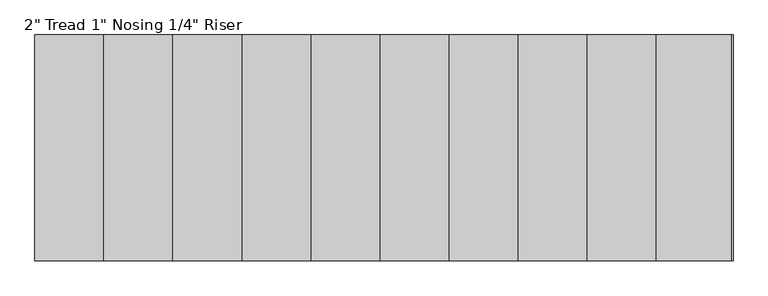
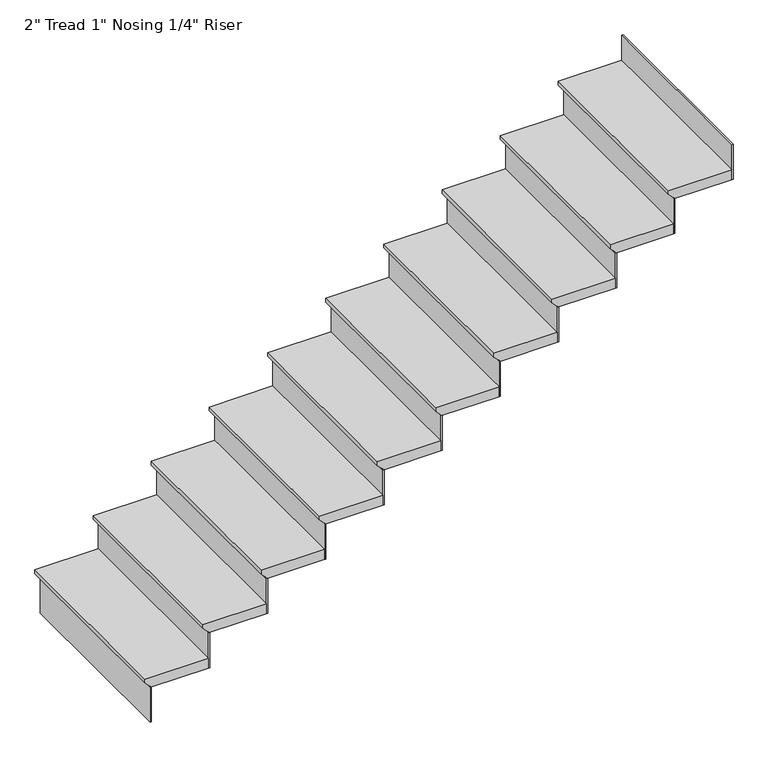
"""IFC4 building model written with IfcOpenShell, lengths in millimetres: stair flight geometry."""

from ifc_helpers import new_model, si_unit, frame, origin, place, context, project, spatial, polyline, outline, extrude, source, transform, mapped, element, save


def stair_flight_d3d59df2(model_context):
    return source(origin(), model_context, "Body", "SweptSolid", [
        extrude(outline(polyline([(1422.4, -12143.9167709), (1422.4, -12448.7167709), (1403.35, -12448.7167709), (1377.95, -12423.3167709), (1371.6, -12423.3167709), (1371.6, -12143.9167709), (1422.4, -12143.9167709)])), frame((0.0, 2766.6362133, 0.0), z_axis=(0.0, 1.0, 0.0), x_axis=(0.0, 0.0, 1.0)), (0.0, 0.0, 1.0), 914.4),
        extrude(outline(polyline([(-12416.9667709, 2766.6362133), (-12423.3167709, 2766.6362133), (-12423.3167709, 3681.0362133), (-12416.9667709, 3681.0362133), (-12416.9667709, 2766.6362133)])), frame((0.0, 0.0, 1193.8), z_axis=(0.0, 0.0, 1.0), x_axis=(1.0, 0.0, 0.0)), (0.0, 0.0, 1.0), 177.8),
        extrude(outline(polyline([(-12137.5667709, 2766.6362133), (-12143.9167709, 2766.6362133), (-12143.9167709, 3681.0362133), (-12137.5667709, 3681.0362133), (-12137.5667709, 2766.6362133)])), frame((0.0, 0.0, 1371.6), z_axis=(0.0, 0.0, 1.0), x_axis=(1.0, 0.0, 0.0)), (0.0, 0.0, 1.0), 177.8),
        extrude(outline(polyline([(1600.2, -11864.5167709), (1600.2, -12169.3167709), (1581.15, -12169.3167709), (1555.75, -12143.9167709), (1549.4, -12143.9167709), (1549.4, -11864.5167709), (1600.2, -11864.5167709)])), frame((0.0, 2766.6362133, 0.0), z_axis=(0.0, 1.0, 0.0), x_axis=(0.0, 0.0, 1.0)), (0.0, 0.0, 1.0), 914.4),
        extrude(outline(polyline([(-11858.1667709, 2766.6362133), (-11864.5167709, 2766.6362133), (-11864.5167709, 3681.0362133), (-11858.1667709, 3681.0362133), (-11858.1667709, 2766.6362133)])), frame((0.0, 0.0, 1549.4), z_axis=(0.0, 0.0, 1.0), x_axis=(1.0, 0.0, 0.0)), (0.0, 0.0, 1.0), 177.8),
        extrude(outline(polyline([(1778.0, -11585.1167709), (1778.0, -11889.9167709), (1758.95, -11889.9167709), (1733.55, -11864.5167709), (1727.2, -11864.5167709), (1727.2, -11585.1167709), (1778.0, -11585.1167709)])), frame((0.0, 2766.6362133, 0.0), z_axis=(0.0, 1.0, 0.0), x_axis=(0.0, 0.0, 1.0)), (0.0, 0.0, 1.0), 914.4),
        extrude(outline(polyline([(-11578.7667709, 2766.6362133), (-11585.1167709, 2766.6362133), (-11585.1167709, 3681.0362133), (-11578.7667709, 3681.0362133), (-11578.7667709, 2766.6362133)])), frame((0.0, 0.0, 1727.2), z_axis=(0.0, 0.0, 1.0), x_axis=(1.0, 0.0, 0.0)), (0.0, 0.0, 1.0), 177.8),
        extrude(outline(polyline([(1955.8, -11305.7167709), (1955.8, -11610.5167709), (1936.75, -11610.5167709), (1911.35, -11585.1167709), (1905.0, -11585.1167709), (1905.0, -11305.7167709), (1955.8, -11305.7167709)])), frame((0.0, 2766.6362133, 0.0), z_axis=(0.0, 1.0, 0.0), x_axis=(0.0, 0.0, 1.0)), (0.0, 0.0, 1.0), 914.4),
        extrude(outline(polyline([(-11299.3667709, 2766.6362133), (-11305.7167709, 2766.6362133), (-11305.7167709, 3681.0362133), (-11299.3667709, 3681.0362133), (-11299.3667709, 2766.6362133)])), frame((0.0, 0.0, 1905.0), z_axis=(0.0, 0.0, 1.0), x_axis=(1.0, 0.0, 0.0)), (0.0, 0.0, 1.0), 177.8),
        extrude(outline(polyline([(2133.6, -11026.3167709), (2133.6, -11331.1167709), (2114.55, -11331.1167709), (2089.15, -11305.7167709), (2082.8, -11305.7167709), (2082.8, -11026.3167709), (2133.6, -11026.3167709)])), frame((0.0, 2766.6362133, 0.0), z_axis=(0.0, 1.0, 0.0), x_axis=(0.0, 0.0, 1.0)), (0.0, 0.0, 1.0), 914.4),
        extrude(outline(polyline([(-11019.9667709, 2766.6362133), (-11026.3167709, 2766.6362133), (-11026.3167709, 3681.0362133), (-11019.9667709, 3681.0362133), (-11019.9667709, 2766.6362133)])), frame((0.0, 0.0, 2082.8), z_axis=(0.0, 0.0, 1.0), x_axis=(1.0, 0.0, 0.0)), (0.0, 0.0, 1.0), 177.8),
        extrude(outline(polyline([(2311.4, -10746.9167709), (2311.4, -11051.7167709), (2292.35, -11051.7167709), (2266.95, -11026.3167709), (2260.6, -11026.3167709), (2260.6, -10746.9167709), (2311.4, -10746.9167709)])), frame((0.0, 2766.6362133, 0.0), z_axis=(0.0, 1.0, 0.0), x_axis=(0.0, 0.0, 1.0)), (0.0, 0.0, 1.0), 914.4),
        extrude(outline(polyline([(-10740.5667709, 2766.6362133), (-10746.9167709, 2766.6362133), (-10746.9167709, 3681.0362133), (-10740.5667709, 3681.0362133), (-10740.5667709, 2766.6362133)])), frame((0.0, 0.0, 2260.6), z_axis=(0.0, 0.0, 1.0), x_axis=(1.0, 0.0, 0.0)), (0.0, 0.0, 1.0), 177.8),
        extrude(outline(polyline([(2489.2, -10467.5167709), (2489.2, -10772.3167709), (2470.15, -10772.3167709), (2444.75, -10746.9167709), (2438.4, -10746.9167709), (2438.4, -10467.5167709), (2489.2, -10467.5167709)])), frame((0.0, 2766.6362133, 0.0), z_axis=(0.0, 1.0, 0.0), x_axis=(0.0, 0.0, 1.0)), (0.0, 0.0, 1.0), 914.4),
        extrude(outline(polyline([(-10461.1667709, 2766.6362133), (-10467.5167709, 2766.6362133), (-10467.5167709, 3681.0362133), (-10461.1667709, 3681.0362133), (-10461.1667709, 2766.6362133)])), frame((0.0, 0.0, 2438.4), z_axis=(0.0, 0.0, 1.0), x_axis=(1.0, 0.0, 0.0)), (0.0, 0.0, 1.0), 177.8),
        extrude(outline(polyline([(2667.0, -10188.1167709), (2667.0, -10492.9167709), (2647.95, -10492.9167709), (2622.55, -10467.5167709), (2616.2, -10467.5167709), (2616.2, -10188.1167709), (2667.0, -10188.1167709)])), frame((0.0, 2766.6362133, 0.0), z_axis=(0.0, 1.0, 0.0), x_axis=(0.0, 0.0, 1.0)), (0.0, 0.0, 1.0), 914.4),
        extrude(outline(polyline([(-10181.7667709, 2766.6362133), (-10188.1167709, 2766.6362133), (-10188.1167709, 3681.0362133), (-10181.7667709, 3681.0362133), (-10181.7667709, 2766.6362133)])), frame((0.0, 0.0, 2616.2), z_axis=(0.0, 0.0, 1.0), x_axis=(1.0, 0.0, 0.0)), (0.0, 0.0, 1.0), 177.8),
        extrude(outline(polyline([(2844.8, -9908.7167709), (2844.8, -10213.5167709), (2825.75, -10213.5167709), (2800.35, -10188.1167709), (2794.0, -10188.1167709), (2794.0, -9908.7167709), (2844.8, -9908.7167709)])), frame((0.0, 2766.6362133, 0.0), z_axis=(0.0, 1.0, 0.0), x_axis=(0.0, 0.0, 1.0)), (0.0, 0.0, 1.0), 914.4),
        extrude(outline(polyline([(-9902.3667709, 2766.6362133), (-9908.7167709, 2766.6362133), (-9908.7167709, 3681.0362133), (-9902.3667709, 3681.0362133), (-9902.3667709, 2766.6362133)])), frame((0.0, 0.0, 2794.0), z_axis=(0.0, 0.0, 1.0), x_axis=(1.0, 0.0, 0.0)), (0.0, 0.0, 1.0), 177.8),
        extrude(outline(polyline([(-9622.9667709, 2766.6362133), (-9629.3167709, 2766.6362133), (-9629.3167709, 3681.0362133), (-9622.9667709, 3681.0362133), (-9622.9667709, 2766.6362133)])), frame((0.0, 0.0, 2971.8), z_axis=(0.0, 0.0, 1.0), x_axis=(1.0, 0.0, 0.0)), (0.0, 0.0, 1.0), 177.8),
        extrude(outline(polyline([(3022.6, -9629.3167709), (3022.6, -9934.1167709), (3003.55, -9934.1167709), (2978.15, -9908.7167709), (2971.8, -9908.7167709), (2971.8, -9629.3167709), (3022.6, -9629.3167709)])), frame((0.0, 2766.6362133, 0.0), z_axis=(0.0, 1.0, 0.0), x_axis=(0.0, 0.0, 1.0)), (0.0, 0.0, 1.0), 914.4),
    ])


if __name__ == "__main__":
    model = new_model("IFC4")
    model_context = context("Model", 3, world=origin())
    ifc_project = project(units=[si_unit("LENGTHUNIT", "METRE", prefix="MILLI")], contexts=[model_context])
    site = spatial("IfcSite", under=ifc_project)
    building = spatial("IfcBuilding", under=site)
    placement = place(None, origin())
    stair_flight_shape = stair_flight_d3d59df2(model_context)
    element("IfcStairFlight", 1, ObjectType="2\" Tread 1\" Nosing 1/4\" Riser", at=placement, inside=building, context=model_context, shape_type="MappedRepresentation", body=[
        mapped(stair_flight_shape, transform((0.0, 0.0, 0.0), x_axis=(1.0, 0.0, 0.0), y_axis=(0.0, 1.0, 0.0), z_axis=(0.0, 0.0, 1.0))),
    ])
    save(model, "model.ifc")
